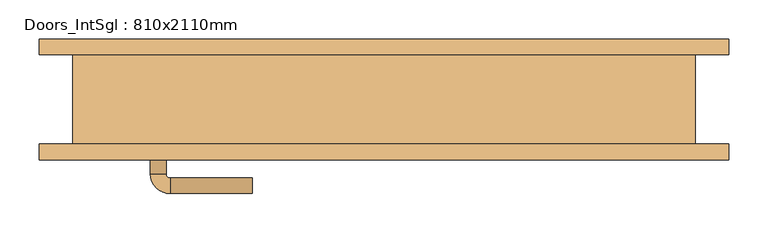
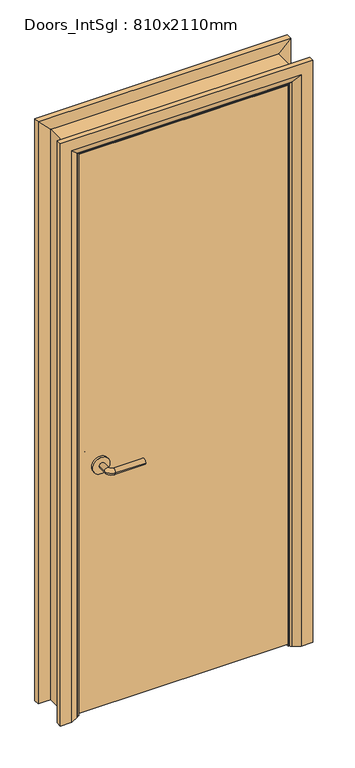
"""IFC4 building model written with IfcOpenShell, lengths in millimetres: door geometry, Doors_IntSgl : 810x2110mm."""

from ifc_helpers import new_model, si_unit, point, frame, frame_2d, origin, place, context, project, spatial, polyline, circle_curve, ellipse_curve, trimmed, segment, composite_curve, outline, extrude, faceted_brep, source, transform, mapped, element, save
from ifc_brep_helpers import plane_surface, cylinder_surface, revolved_surface, advanced_brep


def doors_intsgl_810x2110mm_5608d11f(model_context):
    return source(origin(), model_context, "Body", "SolidModel", [
        advanced_brep(
        [(-298.0, -11.15, 900.0), (-278.0, -11.15, 900.0), (-298.0, 18.85, 900.0), (-278.0, 18.85, 900.0), (-273.0, 23.85, 900.0), (-273.0, 43.85, 900.0), (-168.0, 43.85, 900.0), (-168.0, 23.85, 900.0)],
        [
            (0, 1, circle_curve(frame((-288.0, -11.15, 900.0), z_axis=(0.0, -1.0, 0.0), x_axis=(1.0, 0.0, 0.0)), 10.0)),
            (1, 0, circle_curve(frame((-288.0, -11.15, 900.0), z_axis=(0.0, -1.0, 0.0), x_axis=(1.0, 0.0, 0.0)), 10.0)),
            (0, 2),
            (2, 3, circle_curve(frame((-288.0, 18.85, 900.0), z_axis=(0.0, -1.0, 0.0), x_axis=(1.0, 0.0, 0.0)), 10.0)),
            (3, 1),
            (3, 2, circle_curve(frame((-288.0, 18.85, 900.0), z_axis=(0.0, -1.0, 0.0), x_axis=(1.0, 0.0, 0.0)), 10.0)),
            (4, 3, circle_curve(frame((-273.0, 18.85, 900.0), z_axis=(0.0, 0.0, 1.0), x_axis=(-1.0, 0.0, 0.0)), 5.0)),
            (2, 5, circle_curve(frame((-273.0, 18.85, 900.0), z_axis=(0.0, 0.0, -1.0), x_axis=(-1.0, 0.0, 0.0)), 25.0)),
            (5, 4, circle_curve(frame((-273.0, 33.85, 900.0), z_axis=(-1.0, 0.0, 0.0), x_axis=(0.0, -1.0, 0.0)), 10.0)),
            (4, 5, circle_curve(frame((-273.0, 33.85, 900.0), z_axis=(-1.0, 0.0, 0.0), x_axis=(0.0, -1.0, 0.0)), 10.0)),
            (6, 7, circle_curve(frame((-168.0, 33.85, 900.0), z_axis=(1.0, 0.0, 0.0), x_axis=(0.0, -1.0, 0.0)), 10.0)),
            (7, 6, circle_curve(frame((-168.0, 33.85, 900.0), z_axis=(1.0, 0.0, 0.0), x_axis=(0.0, -1.0, 0.0)), 10.0)),
            (5, 6),
            (7, 4),
        ],
        [
            plane_surface(frame((-288.0, -11.15, 900.0), z_axis=(0.0, -1.0, 0.0), x_axis=(0.0, 0.0, 1.0))),
            cylinder_surface(frame((-288.0, -11.15, 900.0), z_axis=(0.0, -1.0, 0.0), x_axis=(1.0, 0.0, 0.0)), 10.0),
            revolved_surface(trimmed(ellipse_curve(frame((-288.0, 18.85, 900.0), z_axis=(0.0, -1.0, 0.0), x_axis=(1.0, 0.0, 0.0)), 10.0, 10.0), [point((-298.0, 18.85, 900.0))], [point((-278.0, 18.85, 900.0))], True, "CARTESIAN"), (-273.0, 18.85, 900.0), (0.0, 0.0, -1.0)),
            revolved_surface(trimmed(ellipse_curve(frame((-288.0, 18.85, 900.0), z_axis=(0.0, -1.0, 0.0), x_axis=(1.0, 0.0, 0.0)), 10.0, 10.0), [point((-278.0, 18.85, 900.0))], [point((-298.0, 18.85, 900.0))], True, "CARTESIAN"), (-273.0, 18.85, 900.0), (0.0, 0.0, -1.0)),
            plane_surface(frame((-168.0, 33.85, 900.0), z_axis=(1.0, 0.0, 0.0), x_axis=(0.0, 0.0, 1.0))),
            cylinder_surface(frame((-273.0, 33.85, 900.0), z_axis=(-1.0, 0.0, 0.0), x_axis=(0.0, -1.0, 0.0)), 10.0),
        ],
        [
            (0, [[1, 2]]),
            (1, [[-1, 3, 4, 5]]),
            (1, [[-2, -5, 6, -3]]),
            (2, [[7, -4, 8, 9]]),
            (3, [[-8, -6, -7, 10]]),
            (4, [[11, 12]]),
            (5, [[-9, 13, -12, 14]]),
            (5, [[-10, -14, -11, -13]]),
        ],
    ),
        extrude(outline(composite_curve([segment(trimmed(circle_curve(frame_2d((900.0, -290.5)), 30.0), [point((900.0, -320.5))], [point((900.0, -260.5))], False, "CARTESIAN"), True, "CONTINUOUS"), segment(trimmed(circle_curve(frame_2d((900.0, -290.5)), 30.0), [point((900.0, -260.5))], [point((900.0, -320.5))], False, "CARTESIAN"), True, "CONTINUOUS")], self_intersect=False)), frame((0.0, -19.15, 0.0), z_axis=(0.0, 1.0, 0.0), x_axis=(0.0, 0.0, 1.0)), (0.0, 0.0, 1.0), 8.0),
        advanced_brep(
        [(-298.0, -65.15, 900.0), (-278.0, -65.15, 900.0), (-278.0, -95.15, 900.0), (-298.0, -95.15, 900.0), (-273.0, -100.15, 900.0), (-273.0, -120.15, 900.0), (-168.0, -120.15, 900.0), (-168.0, -100.15, 900.0)],
        [
            (0, 1, circle_curve(frame((-288.0, -65.15, 900.0), z_axis=(0.0, 1.0, 0.0), x_axis=(1.0, 0.0, 0.0)), 10.0)),
            (1, 0, circle_curve(frame((-288.0, -65.15, 900.0), z_axis=(0.0, 1.0, 0.0), x_axis=(1.0, 0.0, 0.0)), 10.0)),
            (1, 2),
            (2, 3, circle_curve(frame((-288.0, -95.15, 900.0), z_axis=(0.0, 1.0, 0.0), x_axis=(1.0, 0.0, 0.0)), 10.0)),
            (3, 0),
            (3, 2, circle_curve(frame((-288.0, -95.15, 900.0), z_axis=(0.0, 1.0, 0.0), x_axis=(1.0, 0.0, 0.0)), 10.0)),
            (4, 5, circle_curve(frame((-273.0, -110.15, 900.0), z_axis=(-1.0, 0.0, 0.0), x_axis=(0.0, 1.0, 0.0)), 10.0)),
            (5, 3, circle_curve(frame((-273.0, -95.15, 900.0), z_axis=(0.0, 0.0, -1.0), x_axis=(-1.0, 0.0, 0.0)), 25.0)),
            (2, 4, circle_curve(frame((-273.0, -95.15, 900.0), z_axis=(0.0, 0.0, 1.0), x_axis=(-1.0, 0.0, 0.0)), 5.0)),
            (5, 4, circle_curve(frame((-273.0, -110.15, 900.0), z_axis=(-1.0, 0.0, 0.0), x_axis=(0.0, 1.0, 0.0)), 10.0)),
            (6, 7, circle_curve(frame((-168.0, -110.15, 900.0), z_axis=(1.0, 0.0, 0.0), x_axis=(0.0, 1.0, 0.0)), 10.0)),
            (7, 6, circle_curve(frame((-168.0, -110.15, 900.0), z_axis=(1.0, 0.0, 0.0), x_axis=(0.0, 1.0, 0.0)), 10.0)),
            (4, 7),
            (6, 5),
        ],
        [
            plane_surface(frame((-288.0, -65.15, 900.0), z_axis=(0.0, 1.0, 0.0), x_axis=(0.0, 0.0, 1.0))),
            cylinder_surface(frame((-288.0, -65.15, 900.0), z_axis=(0.0, 1.0, 0.0), x_axis=(1.0, 0.0, 0.0)), 10.0),
            revolved_surface(trimmed(ellipse_curve(frame((-288.0, -95.15, 900.0), z_axis=(0.0, -1.0, 0.0), x_axis=(1.0, 0.0, 0.0)), 10.0, 10.0), [point((-298.0, -95.15, 900.0))], [point((-278.0, -95.15, 900.0))], True, "CARTESIAN"), (-273.0, -95.15, 900.0), (0.0, 0.0, -1.0)),
            revolved_surface(trimmed(ellipse_curve(frame((-288.0, -95.15, 900.0), z_axis=(0.0, -1.0, 0.0), x_axis=(1.0, 0.0, 0.0)), 10.0, 10.0), [point((-278.0, -95.15, 900.0))], [point((-298.0, -95.15, 900.0))], True, "CARTESIAN"), (-273.0, -95.15, 900.0), (0.0, 0.0, -1.0)),
            plane_surface(frame((-168.0, -110.15, 900.0), z_axis=(1.0, 0.0, 0.0), x_axis=(0.0, 0.0, 1.0))),
            cylinder_surface(frame((-273.0, -110.15, 900.0), z_axis=(-1.0, 0.0, 0.0), x_axis=(0.0, 1.0, 0.0)), 10.0),
        ],
        [
            (0, [[1, 2]]),
            (1, [[3, 4, 5, -2]]),
            (1, [[-5, 6, -3, -1]]),
            (2, [[7, 8, -4, 9]]),
            (3, [[10, -9, -6, -8]]),
            (4, [[11, 12]]),
            (5, [[13, -11, 14, -7]]),
            (5, [[-14, -12, -13, -10]]),
        ],
    ),
        extrude(outline(composite_curve([segment(trimmed(circle_curve(frame_2d((900.0, -290.5)), 30.0), [point((900.0, -320.5))], [point((900.0, -260.5))], False, "CARTESIAN"), True, "CONTINUOUS"), segment(trimmed(circle_curve(frame_2d((900.0, -290.5)), 30.0), [point((900.0, -260.5))], [point((900.0, -320.5))], False, "CARTESIAN"), True, "CONTINUOUS")], self_intersect=False)), frame((0.0, -65.15, 0.0), z_axis=(0.0, 1.0, 0.0), x_axis=(0.0, 0.0, 1.0)), (0.0, 0.0, 1.0), 8.0),
        extrude(outline(polyline([(363.0, -19.15), (363.0, -57.15), (-363.0, -57.15), (-363.0, -19.15), (363.0, -19.15)])), frame((0.0, 0.0, 8.0), z_axis=(0.0, 0.0, 1.0), x_axis=(1.0, 0.0, 0.0)), (0.0, 0.0, 1.0), 2060.0),
        advanced_brep(
        [(440.0, -77.15, 0.0), (400.0, -77.15, 0.0), (374.0, -63.15, 0.0), (370.0, -57.15, 0.0), (440.0, -57.15, 0.0), (440.0, -57.15, 2145.0), (440.0, -77.15, 2145.0), (370.0, -57.15, 2075.0), (-370.0, -57.15, 2075.0), (-370.0, -57.15, 0.0), (-440.0, -57.15, 0.0), (-440.0, -57.15, 2145.0), (374.0, -63.15, 2079.0), (400.0, -77.15, 2105.0), (-440.0, -77.15, 2145.0), (-440.0, -77.15, 0.0), (-400.0, -77.15, 0.0), (-400.0, -77.15, 2105.0), (-374.0, -63.15, 2079.0), (-374.0, -63.15, 0.0)],
        [
            (0, 1),
            (1, 2),
            (2, 3, circle_curve(frame((378.0, -56.15, 0.0), z_axis=(0.0, 0.0, -1.0), x_axis=(1.0, 0.0, 0.0)), 8.0622577)),
            (3, 4),
            (4, 0),
            (4, 5),
            (5, 6),
            (6, 0),
            (3, 7),
            (7, 8),
            (8, 9),
            (9, 10),
            (10, 11),
            (11, 5),
            (2, 12),
            (12, 7, ellipse_curve(frame((378.0, -56.15, 2083.0), z_axis=(0.7071067811865475, 0.0, -0.7071067811865475), x_axis=(-0.7071067811865474, 0.0, -0.7071067811865476)), 11.4017543, 8.0622577)),
            (1, 13),
            (13, 12),
            (6, 14),
            (14, 15),
            (15, 16),
            (16, 17),
            (17, 13),
            (11, 14),
            (12, 18),
            (18, 8, ellipse_curve(frame((-378.0, -56.15, 2083.0), z_axis=(0.7071067811865475, 0.0, 0.7071067811865475), x_axis=(0.7071067811865476, 0.0, -0.7071067811865474)), 11.4017543, 8.0622577)),
            (17, 18),
            (15, 10),
            (9, 19, circle_curve(frame((-378.0, -56.15, 0.0), z_axis=(0.0, 0.0, -1.0), x_axis=(-1.0, 0.0, 0.0)), 8.0622577)),
            (19, 16),
            (18, 19),
        ],
        [
            plane_surface(frame((370.0, -57.15, 0.0), z_axis=(0.0, 0.0, -1.0), x_axis=(0.0, 1.0, 0.0))),
            plane_surface(frame((440.0, -77.15, 0.0), z_axis=(1.0, 0.0, 0.0), x_axis=(0.0, 0.0, 1.0))),
            plane_surface(frame((440.0, -57.15, 0.0), z_axis=(0.0, 1.0, 0.0), x_axis=(0.0, 0.0, 1.0))),
            cylinder_surface(frame((378.0, -56.15, 0.0), z_axis=(0.0, 0.0, -1.0), x_axis=(1.0, 0.0, 0.0)), 8.0622577),
            plane_surface(frame((374.0, -63.15, 0.0), z_axis=(-0.4740998230350126, -0.880471099922178, 0.0), x_axis=(0.0, 0.0, 1.0))),
            plane_surface(frame((400.0, -77.15, 0.0), z_axis=(0.0, -1.0, 0.0), x_axis=(0.0, 0.0, 1.0))),
            plane_surface(frame((440.0, -77.15, 2145.0), z_axis=(0.0, 0.0, 1.0), x_axis=(-1.0, 0.0, 0.0))),
            cylinder_surface(frame((370.0, -56.15, 2083.0), z_axis=(1.0, 0.0, 0.0), x_axis=(0.0, 0.0, 1.0)), 8.0622577),
            plane_surface(frame((374.0, -63.15, 2079.0), z_axis=(0.0, -0.8804710999221764, -0.4740998230350154), x_axis=(-1.0, 0.0, 0.0))),
            plane_surface(frame((-370.0, -57.15, 0.0), z_axis=(0.0, 0.0, -1.0), x_axis=(0.0, 1.0, 0.0))),
            plane_surface(frame((-440.0, -77.15, 2145.0), z_axis=(-1.0, 0.0, 0.0), x_axis=(0.0, 0.0, -1.0))),
            cylinder_surface(frame((-378.0, -56.15, 2075.0), z_axis=(0.0, 0.0, 1.0), x_axis=(-1.0, 0.0, 0.0)), 8.0622577),
            plane_surface(frame((-374.0, -63.15, 2079.0), z_axis=(0.47409982303501824, -0.8804710999221749, 0.0), x_axis=(0.0, 0.0, -1.0))),
        ],
        [
            (0, [[1, 2, 3, 4, 5]]),
            (1, [[6, 7, 8, -5]]),
            (2, [[9, 10, 11, 12, 13, 14, -6, -4]]),
            (3, [[15, 16, -9, -3]]),
            (4, [[17, 18, -15, -2]]),
            (5, [[-8, 19, 20, 21, 22, 23, -17, -1]]),
            (6, [[-14, 24, -19, -7]]),
            (7, [[25, 26, -10, -16]]),
            (8, [[-23, 27, -25, -18]]),
            (9, [[28, -12, 29, 30, -21]]),
            (10, [[-13, -28, -20, -24]]),
            (11, [[31, -29, -11, -26]]),
            (12, [[-22, -30, -31, -27]]),
        ],
    ),
        extrude(outline(polyline([(0.0, -346.0), (2051.0, -346.0), (2051.0, 346.0), (0.0, 346.0), (0.0, 365.0), (2070.0, 365.0), (2070.0, -365.0), (0.0, -365.0), (0.0, -346.0)])), frame((0.0, -17.15, 0.0), z_axis=(0.0, 1.0, 0.0), x_axis=(0.0, 0.0, 1.0)), (0.0, 0.0, 1.0), 32.0),
        advanced_brep(
        [(-440.0, 77.15, 0.0), (-400.0, 77.15, 0.0), (-374.0, 63.15, 0.0), (-370.0, 57.15, 0.0), (-440.0, 57.15, 0.0), (-440.0, 57.15, 2145.0), (-440.0, 77.15, 2145.0), (-370.0, 57.15, 2075.0), (-374.0, 63.15, 2079.0), (-400.0, 77.15, 2105.0), (440.0, 57.15, 2145.0), (440.0, 77.15, 2145.0), (370.0, 57.15, 2075.0), (374.0, 63.15, 2079.0), (400.0, 77.15, 2105.0), (440.0, 77.15, 0.0), (440.0, 57.15, 0.0), (370.0, 57.15, 0.0), (374.0, 63.15, 0.0), (400.0, 77.15, 0.0)],
        [
            (0, 1),
            (1, 2),
            (2, 3, circle_curve(frame((-378.0, 56.15, 0.0), z_axis=(0.0, 0.0, -1.0), x_axis=(-1.0, 0.0, 0.0)), 8.0622577)),
            (3, 4),
            (4, 0),
            (4, 5),
            (5, 6),
            (6, 0),
            (3, 7),
            (7, 5),
            (2, 8),
            (8, 7, ellipse_curve(frame((-378.0, 56.15, 2083.0), z_axis=(-0.7071067811865475, 0.0, -0.7071067811865475), x_axis=(0.7071067811865474, 0.0, -0.7071067811865476)), 11.4017543, 8.0622577)),
            (1, 9),
            (9, 8),
            (6, 9),
            (5, 10),
            (10, 11),
            (11, 6),
            (7, 12),
            (12, 10),
            (8, 13),
            (13, 12, ellipse_curve(frame((378.0, 56.15, 2083.0), z_axis=(-0.7071067811865475, 0.0, 0.7071067811865475), x_axis=(-0.7071067811865476, 0.0, -0.7071067811865474)), 11.4017543, 8.0622577)),
            (9, 14),
            (14, 13),
            (11, 14),
            (15, 16),
            (16, 17),
            (17, 18, circle_curve(frame((378.0, 56.15, 0.0), z_axis=(0.0, 0.0, -1.0), x_axis=(1.0, 0.0, 0.0)), 8.0622577)),
            (18, 19),
            (19, 15),
            (10, 16),
            (15, 11),
            (12, 17),
            (13, 18),
            (14, 19),
        ],
        [
            plane_surface(frame((-370.0, 129.9510989, 0.0), z_axis=(0.0, 0.0, -1.0), x_axis=(1.0, 0.0, 0.0))),
            plane_surface(frame((-440.0, 77.15, 0.0), z_axis=(-1.0, 0.0, 0.0), x_axis=(0.0, 0.0, 1.0))),
            plane_surface(frame((-440.0, 57.15, 0.0), z_axis=(0.0, -1.0, 0.0), x_axis=(0.0, 0.0, 1.0))),
            cylinder_surface(frame((-378.0, 56.15, 0.0), z_axis=(0.0, 0.0, -1.0), x_axis=(-1.0, 0.0, 0.0)), 8.0622577),
            plane_surface(frame((-374.0, 63.15, 0.0), z_axis=(0.4740998230350183, 0.8804710999221749, 0.0), x_axis=(0.0, 0.0, 1.0))),
            plane_surface(frame((-400.0, 77.15, 0.0), z_axis=(0.0, 1.0, 0.0), x_axis=(0.0, 0.0, 1.0))),
            plane_surface(frame((-440.0, 77.15, 2145.0), z_axis=(0.0, 0.0, 1.0), x_axis=(1.0, 0.0, 0.0))),
            plane_surface(frame((-440.0, 57.15, 2145.0), z_axis=(0.0, -1.0, 0.0), x_axis=(1.0, 0.0, 0.0))),
            cylinder_surface(frame((-370.0, 56.15, 2083.0), z_axis=(-1.0, 0.0, 0.0), x_axis=(0.0, 0.0, 1.0)), 8.0622577),
            plane_surface(frame((-374.0, 63.15, 2079.0), z_axis=(0.0, 0.8804710999221749, -0.4740998230350183), x_axis=(1.0, 0.0, 0.0))),
            plane_surface(frame((-400.0, 77.15, 2105.0), z_axis=(0.0, 1.0, 0.0), x_axis=(1.0, 0.0, 0.0))),
            plane_surface(frame((370.0, 129.9510989, 0.0), z_axis=(0.0, 0.0, -1.0), x_axis=(-1.0, 0.0, 0.0))),
            plane_surface(frame((440.0, 77.15, 2145.0), z_axis=(1.0, 0.0, 0.0), x_axis=(0.0, 0.0, -1.0))),
            plane_surface(frame((440.0, 57.15, 2145.0), z_axis=(0.0, -1.0, 0.0), x_axis=(0.0, 0.0, -1.0))),
            cylinder_surface(frame((378.0, 56.15, 2075.0), z_axis=(0.0, 0.0, 1.0), x_axis=(1.0, 0.0, 0.0)), 8.0622577),
            plane_surface(frame((374.0, 63.15, 2079.0), z_axis=(-0.4740998230350183, 0.8804710999221749, 0.0), x_axis=(0.0, 0.0, -1.0))),
            plane_surface(frame((400.0, 77.15, 2105.0), z_axis=(0.0, 1.0, 0.0), x_axis=(0.0, 0.0, -1.0))),
        ],
        [
            (0, [[1, 2, 3, 4, 5]]),
            (1, [[6, 7, 8, -5]]),
            (2, [[9, 10, -6, -4]]),
            (3, [[11, 12, -9, -3]]),
            (4, [[13, 14, -11, -2]]),
            (5, [[-8, 15, -13, -1]]),
            (6, [[16, 17, 18, -7]]),
            (7, [[19, 20, -16, -10]]),
            (8, [[21, 22, -19, -12]]),
            (9, [[23, 24, -21, -14]]),
            (10, [[-18, 25, -23, -15]]),
            (11, [[26, 27, 28, 29, 30]]),
            (12, [[31, -26, 32, -17]]),
            (13, [[33, -27, -31, -20]]),
            (14, [[34, -28, -33, -22]]),
            (15, [[35, -29, -34, -24]]),
            (16, [[-32, -30, -35, -25]]),
        ],
    ),
        faceted_brep([(-365.0, -57.15, 0.0), (-397.0, -57.15, 0.0), (-397.0, 57.15, 0.0), (-365.0, 57.15, 0.0), (-365.0, 57.15, 2070.0), (-365.0, -57.15, 2070.0), (-397.0, 57.15, 2102.0), (-397.0, -57.15, 2102.0), (365.0, 57.15, 2070.0), (365.0, -57.15, 2070.0), (397.0, 57.15, 2102.0), (397.0, -57.15, 2102.0), (365.0, -57.15, 0.0), (365.0, 57.15, 0.0), (397.0, 57.15, 0.0), (397.0, -57.15, 0.0)], [[[0, 1, 2, 3]], [[3, 4, 5, 0]], [[2, 6, 4, 3]], [[1, 7, 6, 2]], [[0, 5, 7, 1]], [[4, 8, 9, 5]], [[6, 10, 8, 4]], [[7, 11, 10, 6]], [[5, 9, 11, 7]], [[12, 13, 14, 15]], [[8, 13, 12, 9]], [[10, 14, 13, 8]], [[11, 15, 14, 10]], [[9, 12, 15, 11]]]),
    ])


if __name__ == "__main__":
    model = new_model("IFC4")
    model_context = context("Model", 3, world=origin())
    ifc_project = project(units=[si_unit("LENGTHUNIT", "METRE", prefix="MILLI")], contexts=[model_context])
    site = spatial("IfcSite", under=ifc_project)
    building = spatial("IfcBuilding", under=site)
    placement = place(None, origin())
    doors_intsgl_810x2110mm_shape = doors_intsgl_810x2110mm_5608d11f(model_context)
    element("IfcDoor", 1, ObjectType="Doors_IntSgl : 810x2110mm", at=placement, inside=building, context=model_context, shape_type="MappedRepresentation", body=[
        mapped(doors_intsgl_810x2110mm_shape, transform((0.0, 0.0, 0.0), x_axis=(1.0, 0.0, 0.0), y_axis=(0.0, 1.0, 0.0), z_axis=(0.0, 0.0, 1.0))),
    ])
    save(model, "model.ifc")

# Revit data of these elements
# Type "Doors_IntSgl : 810x2110mm"
#   Construction Type Id = "MDOOR"
#   Type Mark = "42"
#   Type Comments = "Internal Single"
#   Operation = "SingleSwingRight"
#   Manufacturer = "Revit"
#   Keynote = "L20"
#   Description = "Internal Single Door"
#   Analytic Construction = "Metal"
#   UnderCut = 0' - 0.31496"
#   Tolerance = 0' - 0.07874"
#   Thickness = 0' - 1.49606"
#   Thermal Resistance (R) = 0.270117 (m²·K)/W
#   Structural Tolerance = 0' - 0.31496"
#   StopDepth = 0' - 1.25984"
#   Stop Thickness = 0' - 0.74803"
#   Rough Width = 2' - 7.88976"
#   Rough Height = 6' - 11.07087"
#   Height to Top Lock Rail = 3' - 3.37008"
#   Heat Transfer Coefficient (U) = 3.7021 W/(m²·K)
#   Handle Z Distance = 2' - 11.43307"
#   Handle X Distance = 0' - 2.95276"
#   Frame Thickness = 0' - 1.25984"
#   Door Panel Width = 2' - 4.58268"
#   Door Panel Thickness = 0' - 1.49606"
#   Door Panel Offset = 0' - 0"
#   Height = 6' - 11.07087"
#   Width = 2' - 7.88976"
#   Door Panel Height = 6' - 9.10236"
#   Architrave Setback = 0' - 0.19685"
#   Define Thermal Properties by = 1
#   Vis - Ironmongery = yes
#   Material Ironmongery = Door - Handle
#   Material Frame = Door - Frame/Mullion (1)
#   Material Door = Door - Panel
#   Material Architrave = Door - Architrave
#   Visual Light Transmittance = 0
#   Solar Heat Gain Coefficient = 0
#   Function = (empty or 0)
#   Wall Closure = (empty or 0)
# Element 1 (IfcDoor, "Doors_IntSgl : 810x2110mm")
#   Materials on its faces: "Door - Architrave", "Door - Handle", "Door - Frame/Mullion (1)", "Door - Panel"
# Materials
#   "Door - Handle": colour RGB 17 17 17, transparency 0, Keynote = "P21", Cost = 0
#   "Door - Frame/Mullion (1)": class "Wood", colour RGB 212 179 113, transparency 0, Keynote = "L20", Cost = 0
#   "Door - Panel": class "Wood", colour RGB 210 159 95, transparency 0, Keynote = "L20", Cost = 0
#   "Door - Architrave": class "Wood", colour RGB 154 90 5, transparency 0, Keynote = "P20", Cost = 0
